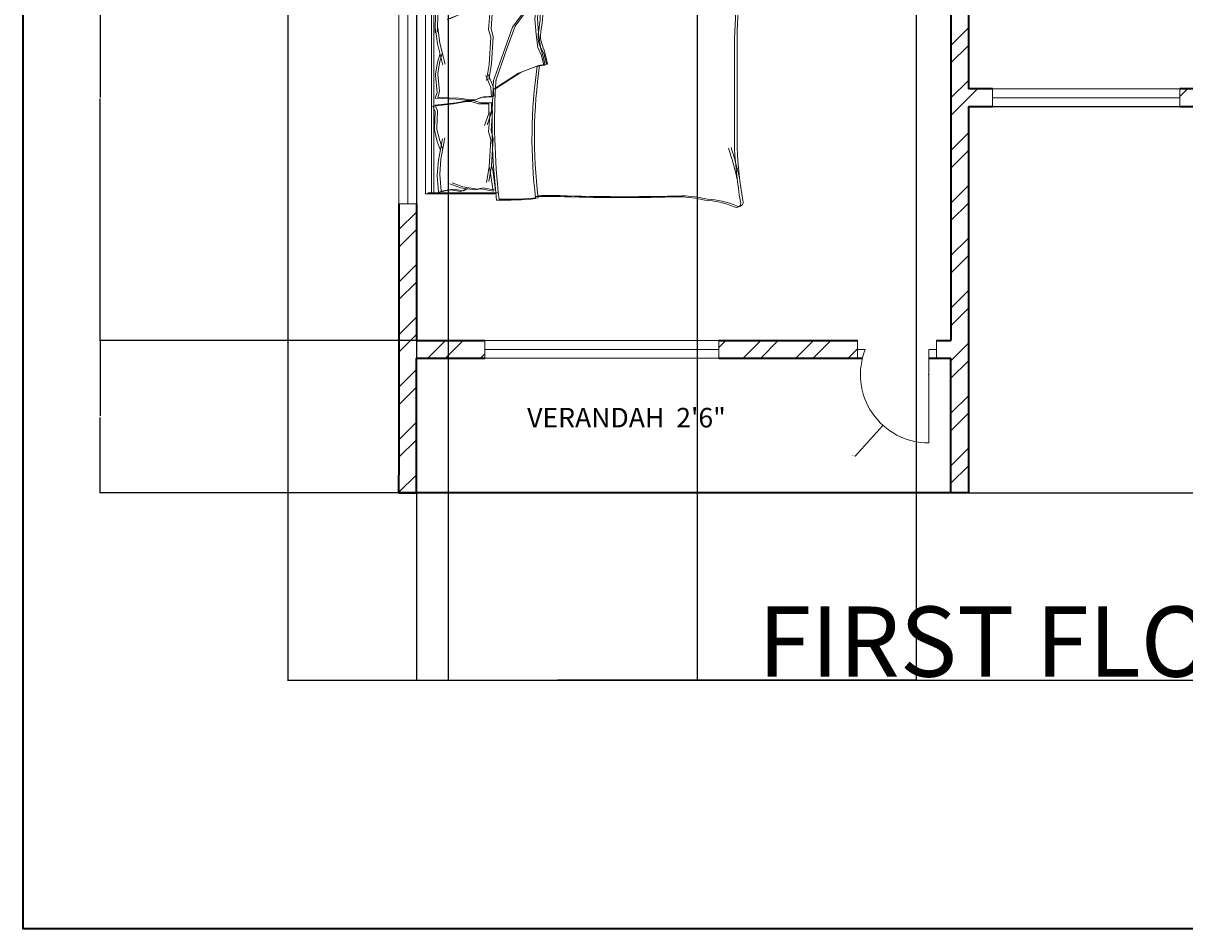
# Model space of a CAD drawing. Units: inches. Extents: x 2008 to 2657, y 1077 to 2165.
# Tile 1 of 16: x 2008 to 2306, y 1077 to 1309. Entities that reach past the tile are written whole.
import ezdxf

# ---------------------------------------------------------------- set-up
doc = ezdxf.new("R2010")
doc.units = ezdxf.units.IN
for name, color, linetype, lineweight in [('A-ANNO-DIMS', 2, 'Continuous', 18), ('A-ANNO-TITL', 7, 'Continuous', 35), ('A-ANNO-TTLB', 7, 'Continuous', 35), ('A-AREA-IDEN', 4, 'Continuous', 18), ('A-DOOR', 11, 'Continuous', 18), ('A-FURN', 8, 'Continuous', 13), ('A-GLAZ', 191, 'Continuous', 18), ('A-WALL', 7, 'Continuous', 35)]:
    doc.layers.add(name, color=color, linetype=linetype, lineweight=lineweight)
doc.layers.add('A-WALL-PATT', color=30, linetype='Continuous', lineweight=13, true_color=0xf8991e)
doc.styles.get("Standard").update_dxf_attribs({"font": 'arial.ttf'})
doc.dimstyles.get("Standard").update_dxf_attribs({"dimtxt": 0.18, "dimasz": 0.18, "dimexe": 0.18, "dimexo": 0.0625, "dimgap": 0.09, "dimtad": 0, "dimtih": 1, "dimtoh": 1, "dimdec": 4, "dimzin": 0, "dimdsep": 46, "dimtxsty": 'Standard', "dimcen": 0.09, "dimadec": 0, "dimazin": 0, "dimtfac": 1, "dimtdec": 4, "dimtofl": 0, "dimtmove": 0, "dimatfit": 3, "dimfxl": 1, "dimtolj": 1, "dimtzin": 0, "dimarcsym": 0})

# ---------------------------------------------------------------- blocks, each defined once
blk = doc.blocks.new('BED-DOUBLE')
for p, q in [((0, 51.49), (0.64, 51.49)), ((0, 3.48), (0, 51.49)), ((0, 51.27), (26.61, 51.27)), ((0, 51.27), (26.61, 51.27)), ((0.64, 51.49), (27.25, 51.49)), ((0.64, 51.49), (27.25, 51.49)), ((1.53, 3.48), (1.53, 51.27)), ((1.53, 3.48), (1.53, 51.27)), ((2.17, 3.7), (2.17, 51.49)), ((2.17, 3.7), (2.17, 51.49)), ((16.57, 50.7), (13.43, 49.92)), ((16.57, 50.7), (13.43, 49.92)), ((17.21, 50.93), (14.07, 50.15)), ((17.21, 50.93), (14.07, 50.15)), ((16.17, 45.57), (16.57, 50.7)), ((16.17, 45.57), (16.57, 50.7)), ((16.81, 45.8), (17.21, 50.93)), ((16.81, 45.8), (17.21, 50.93)), ((27.75, 52.87), (24.5, 49.16)), ((27.75, 52.87), (24.5, 49.16)), ((28.39, 53.1), (25.14, 49.39)), ((28.39, 53.1), (25.14, 49.39)), ((29.49, 52.95), (27.75, 52.87, 3.87)), ((29.49, 52.95), (27.75, 52.87, 3.87)), ((28.37, 51.33), (27.75, 52.87)), ((28.37, 51.33), (27.75, 52.87)), ((28.06, 48.23), (28.37, 51.33)), ((28.06, 48.23), (28.37, 51.33)), ((30.13, 53.18), (28.39, 53.1, 3.87)), ((30.13, 53.18), (28.39, 53.1, 3.87)), ((29, 51.56), (28.39, 53.1)), ((29, 51.56), (28.39, 53.1)), ((28.7, 48.46), (29, 51.56)), ((28.7, 48.46), (29, 51.56)), ((2.56, 50.11), (2.46, 44.71)), ((2.56, 50.11), (2.46, 44.71)), ((2.56, 50.11), (5.77, 49.73)), ((2.56, 50.11), (5.77, 49.73)), ((3.2, 50.34), (3.1, 44.94)), ((3.2, 50.34), (3.1, 44.94)), ((3.2, 50.34), (6.41, 49.96)), ((3.2, 50.34), (6.41, 49.96)), ((8.26, 49.31), (5.58, 48.13)), ((8.26, 49.31), (5.58, 48.13)), ((5.77, 49.73), (8.34, 50.33)), ((5.77, 49.73), (8.34, 50.33)), ((8.9, 49.54), (6.22, 48.36)), ((8.9, 49.54), (6.22, 48.36)), ((6.41, 49.96), (8.98, 50.56)), ((6.41, 49.96), (8.98, 50.56)), ((11.83, 50.11), (8.26, 49.31)), ((11.83, 50.11), (8.26, 49.31)), ((8.34, 50.33), (9.38, 49.82)), ((8.34, 50.33), (9.38, 49.81)), ((12.47, 50.34), (8.9, 49.54)), ((12.47, 50.34), (8.9, 49.54)), ((8.98, 50.56), (10.02, 50.04)), ((8.98, 50.56), (10.02, 50.04)), ((13.43, 49.92), (11.83, 50.11)), ((13.43, 49.92), (11.83, 50.11)), ((14.07, 50.15), (12.47, 50.34)), ((14.07, 50.15), (12.47, 50.34)), ((24.5, 49.16), (22.33, 46.22)), ((24.5, 49.16), (22.33, 46.22)), ((25.14, 49.39), (22.97, 46.45)), ((25.14, 49.39), (22.97, 46.45)), ((28.37, 44.36), (28.06, 48.23)), ((28.37, 44.36), (28.06, 48.23)), ((29, 44.59), (28.7, 48.46)), ((29, 44.59), (28.7, 48.46)), ((2.46, 44.71), (2.54, 45.71)), ((2.46, 44.71), (2.54, 45.71)), ((2.54, 45.71), (3.07, 41.91)), ((2.54, 45.71), (3.07, 41.91)), ((3.1, 44.94), (3.18, 45.94)), ((3.1, 44.94), (3.18, 45.94)), ((3.18, 45.94), (3.71, 42.14)), ((3.18, 45.94), (3.71, 42.14)), ((16.73, 43.61), (16.17, 45.57)), ((16.73, 43.61), (16.17, 45.57)), ((17.37, 43.84), (16.81, 45.8)), ((17.37, 43.83), (16.81, 45.8)), ((22.33, 46.22), (20.32, 40.64)), ((22.33, 46.22), (20.32, 40.64)), ((22.97, 46.45), (20.96, 40.87)), ((22.97, 46.45), (20.96, 40.87)), ((3.07, 41.91), (4.42, 36.5)), ((3.07, 41.91), (4.42, 36.5)), ((3.71, 42.14), (5.06, 36.72)), ((3.71, 42.14), (5.06, 36.72)), ((16.3, 36.6), (16.73, 43.61)), ((16.3, 36.6), (16.73, 43.61)), ((16.93, 36.83), (17.37, 43.84)), ((16.93, 36.82), (17.37, 43.83)), ((28.83, 40.95), (28.37, 44.36)), ((28.83, 40.95), (28.37, 44.36)), ((29.47, 41.18), (29, 44.59)), ((29.47, 41.18), (29, 44.59)), ((3.67, 39.2), (3.08, 37.14)), ((3.67, 39.2), (3.08, 37.14)), ((4.31, 39.43), (3.72, 37.36)), ((4.31, 39.43), (3.72, 37.36)), ((20.32, 40.64), (17.38, 32.31)), ((20.32, 40.64), (17.38, 32.31)), ((20.96, 40.87), (18.02, 32.54)), ((20.96, 40.87), (18.02, 32.53)), ((29.76, 38.94), (28.83, 40.95)), ((29.76, 38.94), (28.83, 40.95)), ((30.4, 39.17), (29.47, 41.18)), ((30.4, 39.17), (29.47, 41.18)), ((30.38, 36.46), (29.76, 38.94)), ((30.38, 36.46), (29.76, 38.94)), ((31.02, 36.69), (30.4, 39.17)), ((31.02, 36.69), (30.4, 39.17)), ((79.25, 15.06), (79.25, 39.68)), ((79.25, 15.06), (79.25, 39.68)), ((79.88, 15.29), (79.88, 39.91)), ((79.88, 15.29), (79.88, 39.91)), ((3.08, 37.14), (2.54, 34.21)), ((3.08, 37.14), (2.54, 34.2)), ((3.72, 37.36), (3.18, 34.43)), ((3.72, 37.36), (3.18, 34.43)), ((15.63, 32.56), (16.3, 36.6)), ((15.63, 32.56), (16.3, 36.6)), ((16.27, 32.79), (16.93, 36.83)), ((16.27, 32.79), (16.93, 36.82)), ((23.88, 34.45), (28.37, 36.15)), ((23.88, 34.45), (28.37, 36.15)), ((24.52, 34.68), (29, 36.38)), ((24.52, 34.68), (29, 36.38)), ((28.37, 36.15), (30.38, 36.46)), ((28.37, 36.15), (30.38, 36.46)), ((29, 36.38), (31.02, 36.69)), ((29, 36.38), (31.02, 36.69)), ((2.54, 34.21), (2.56, 33.88)), ((2.54, 34.2), (2.56, 33.88)), ((2.56, 33.88), (2.98, 29.46)), ((2.56, 33.88), (2.98, 29.46)), ((3.18, 34.43), (3.2, 34.11)), ((3.18, 34.43), (3.2, 34.11)), ((3.2, 34.11), (3.62, 29.68)), ((3.2, 34.11), (3.62, 29.68)), ((16.74, 30.75), (15.45, 33.82)), ((16.74, 30.75), (15.45, 33.82)), ((17.38, 30.98), (16.09, 34.05)), ((17.38, 30.98), (16.09, 34.05)), ((17.38, 30.26), (23.88, 34.45)), ((17.38, 30.26), (23.88, 34.45)), ((18.02, 30.49), (24.52, 34.68)), ((18.02, 30.49), (24.52, 34.68)), ((16.89, 28.3), (16.74, 30.75)), ((16.89, 28.3), (16.74, 30.75)), ((17.53, 28.53), (17.38, 30.98)), ((17.53, 28.53), (17.38, 30.98)), ((2.98, 29.46), (2.49, 27.98)), ((2.98, 29.46), (2.49, 27.98)), ((2.49, 27.98), (7.87, 27.73)), ((2.49, 27.98), (7.87, 27.73)), ((3.62, 29.68), (3.13, 28.21)), ((3.62, 29.68), (3.13, 28.21)), ((3.13, 28.21), (8.51, 27.96)), ((3.13, 28.21), (8.51, 27.96)), ((7.22, 26.56), (10.4, 27.14)), ((7.22, 26.56), (10.4, 27.14)), ((7.86, 26.79), (11.04, 27.37)), ((7.86, 26.79), (11.04, 27.37)), ((7.87, 27.73), (11.08, 27.36)), ((7.87, 27.73), (11.08, 27.36)), ((8.51, 27.96), (11.72, 27.58)), ((8.51, 27.96), (11.72, 27.58)), ((10.4, 27.14), (11.7, 27.14)), ((10.4, 27.14), (11.7, 27.14)), ((11.04, 27.37), (12.34, 27.37)), ((11.04, 27.37), (12.34, 27.37)), ((11.08, 27.36), (12.38, 27.44)), ((11.08, 27.36), (12.38, 27.44)), ((11.7, 27.14), (13.58, 26.56)), ((11.7, 27.14), (13.58, 26.56)), ((11.72, 27.58), (13.02, 27.66)), ((11.72, 27.58), (13.02, 27.66)), ((12.34, 27.37), (14.22, 26.79)), ((12.34, 27.37), (14.22, 26.79)), ((12.38, 27.44), (14.22, 28.13)), ((12.38, 27.44), (14.22, 28.13)), ((13.02, 27.66), (14.86, 28.36)), ((13.02, 27.66), (14.86, 28.36)), ((14.22, 28.13), (16.89, 28.3)), ((14.22, 28.13), (16.89, 28.3)), ((14.86, 28.36), (17.53, 28.53)), ((14.86, 28.36), (17.53, 28.53)), ((1.87, 25.98), (7.22, 26.56)), ((1.87, 25.98), (7.22, 26.56)), ((2.45, 24.54), (1.87, 25.98)), ((2.45, 24.54), (1.87, 25.98)), ((2.3, 20.09), (2.45, 24.54)), ((2.3, 20.09), (2.45, 24.54)), ((2.51, 26.21), (7.86, 26.79)), ((2.51, 26.21), (7.86, 26.79)), ((3.09, 24.77), (2.51, 26.21)), ((3.09, 24.77), (2.51, 26.21)), ((2.94, 20.32), (3.09, 24.77)), ((2.94, 20.32), (3.09, 24.77)), ((13.58, 26.56), (16.26, 26.56)), ((13.58, 26.56), (16.26, 26.56)), ((14.22, 26.79), (16.9, 26.79)), ((14.22, 26.79), (16.9, 26.79)), ((16.26, 24.1), (15.17, 20.96)), ((16.26, 24.1), (15.17, 20.96)), ((16.9, 24.33), (15.81, 21.19)), ((16.9, 24.33), (15.81, 21.19)), ((16.17, 19.38), (16.57, 24.52)), ((16.17, 19.38), (16.57, 24.52)), ((16.26, 26.56), (16.26, 24.1)), ((16.26, 26.56), (16.26, 24.1)), ((16.81, 19.61), (17.21, 24.74)), ((16.81, 19.61), (17.21, 24.74)), ((16.9, 26.79), (16.9, 24.33)), ((16.9, 26.79), (16.9, 24.33)), ((2.3, 19.77), (2.3, 20.09)), ((2.3, 19.77), (2.3, 20.09)), ((3.03, 16.88), (2.3, 19.77)), ((3.03, 16.88), (2.3, 19.77)), ((2.94, 20), (2.94, 20.32)), ((2.94, 20), (2.94, 20.32)), ((3.67, 17.11), (2.94, 20)), ((3.67, 17.11), (2.94, 20)), ((16.73, 17.42), (16.17, 19.38)), ((16.73, 17.42), (16.17, 19.38)), ((17.37, 17.65), (16.81, 19.61)), ((17.37, 17.65), (16.81, 19.61)), ((3.75, 14.86), (3.03, 16.88)), ((3.75, 14.86), (3.03, 16.88)), ((3.32, 12.11), (4.33, 17.6)), ((3.32, 12.11), (4.33, 17.6)), ((4.39, 15.08), (3.67, 17.11)), ((4.39, 15.08), (3.67, 17.11)), ((3.96, 12.34), (4.97, 17.83)), ((3.96, 12.34), (4.97, 17.83)), ((16.3, 10.41), (16.73, 17.42)), ((16.3, 10.41), (16.73, 17.42)), ((16.93, 10.64), (17.37, 17.65)), ((16.93, 10.64), (17.37, 17.65)), ((3.03, 8.29), (3.32, 12.11)), ((3.03, 8.29), (3.32, 12.11)), ((3.67, 8.51), (3.96, 12.34)), ((3.67, 8.51), (3.96, 12.34)), ((15.63, 6.38), (16.3, 10.41)), ((15.63, 6.38), (16.3, 10.41)), ((16.27, 6.61), (16.93, 10.64)), ((16.27, 6.61), (16.93, 10.64)), ((16.3, 10.41), (16.62, 9.28)), ((16.3, 10.41), (16.62, 9.28)), ((16.62, 9.28), (17.34, 4.18)), ((16.62, 9.28), (17.34, 4.18)), ((16.93, 10.64), (17.26, 9.51)), ((16.93, 10.64), (17.26, 9.51)), ((17.26, 9.51), (17.98, 4.41)), ((17.26, 9.51), (17.98, 4.41)), ((3.01, 8.18), (3.03, 8.29)), ((3.01, 8.18), (3.03, 8.29)), ((3.34, 3.9), (3.01, 8.18)), ((3.34, 3.9), (3.01, 8.18)), ((3.65, 8.41), (3.67, 8.51)), ((3.65, 8.41), (3.67, 8.51)), ((3.98, 4.13), (3.65, 8.41)), ((3.98, 4.13), (3.65, 8.41)), ((8.96, 5.05), (6.21, 6.06)), ((8.96, 5.05), (6.21, 6.06)), ((9.59, 5.28), (6.85, 6.29)), ((9.59, 5.28), (6.85, 6.29)), ((18.11, 3.48), (0, 3.48)), ((18.11, 3.48), (0, 3.48)), ((18.75, 3.7), (0.64, 3.7)), ((18.75, 3.7), (0.64, 3.7)), ((3.32, 3.9), (6.5, 4.47)), ((3.32, 3.89), (6.5, 4.47)), ((3.96, 4.12), (7.14, 4.7)), ((3.96, 4.12), (7.14, 4.7)), ((6.5, 4.47), (9.1, 4.04)), ((6.5, 4.47), (9.1, 4.04)), ((7.14, 4.7), (9.74, 4.27)), ((7.14, 4.7), (9.74, 4.27)), ((12.57, 4.47), (8.96, 5.05)), ((12.57, 4.47), (8.96, 5.05)), ((9.1, 4.04), (10.11, 4.62)), ((9.1, 4.04), (10.11, 4.62)), ((13.21, 4.7), (9.59, 5.28)), ((13.21, 4.7), (9.59, 5.28)), ((9.74, 4.27), (10.75, 4.85)), ((9.74, 4.27), (10.75, 4.85)), ((14.16, 4.76), (12.57, 4.47)), ((14.16, 4.76), (12.57, 4.47)), ((14.8, 4.99), (13.21, 4.7)), ((14.8, 4.99), (13.21, 4.7)), ((17.34, 4.18), (14.16, 4.76)), ((17.34, 4.18), (14.16, 4.76)), ((17.98, 4.41), (14.8, 4.99)), ((17.98, 4.41), (14.8, 4.99))]:
    blk.add_line(p, q)
for centre, radius, start, end in [((68.67, 76.16), 23.07, 267.4714, 296.4681), ((68.67, 76.16), 23.07, 267.4714, 296.4681), ((69.31, 76.39), 23.07, 267.4714, 296.4681), ((69.31, 76.39), 23.07, 267.4714, 296.4681), ((78.87, 54.41), 1.1, 332.6588, 86.02), ((78.87, 54.41), 1.1, 332.6588, 86.02), ((212.28, 41.15), 133.04, 174.4998, 180.6351), ((212.28, 41.15), 133.04, 174.4998, 180.6351), ((79.51, 54.64), 1.1, 332.6588, 86.02), ((79.51, 54.64), 1.1, 332.6588, 86.02), ((212.92, 41.38), 133.04, 174.4998, 180.6351), ((212.92, 41.38), 133.04, 174.4998, 180.6351), ((-6.66, 51.33), 36.18, 349.8763, 2.5657), ((-6.66, 51.33), 36.18, 349.8763, 2.5657), ((36.32, 182.27), 129.5, 266.9791, 273.8365), ((36.32, 182.27), 129.5, 266.9791, 273.8365), ((-6.02, 51.56), 36.18, 349.8763, 2.5657), ((-6.02, 51.56), 36.18, 349.8763, 2.5657), ((36.95, 182.49), 129.5, 266.9791, 273.8365), ((36.95, 182.49), 129.5, 266.9791, 273.8365), ((67.82, -4508.74), 4561.86, 90.00217, 90.28689), ((67.82, -4508.74), 4561.86, 90.00217, 90.28689), ((68.46, -4508.51), 4561.86, 90.00217, 90.28689), ((68.46, -4508.51), 4561.86, 90.00217, 90.28689), ((35.07, 43.74), 6.22, 168.6608, 203.7384), ((35.07, 43.74), 6.22, 168.6608, 203.7384), ((35.71, 43.97), 6.22, 168.6608, 203.7384), ((35.71, 43.97), 6.22, 168.6608, 203.7384), ((1.48, 31.15), 29.65, 10.6617, 19.8806), ((1.48, 31.15), 29.65, 10.6617, 19.8806), ((2.12, 31.38), 29.65, 10.6617, 19.8806), ((2.12, 31.38), 29.65, 10.6617, 19.8806), ((156.32, 17.76), 129.02, 171.7845, 186.9006), ((156.32, 17.76), 129.02, 171.7845, 186.9006), ((156.96, 17.98), 129.02, 171.7845, 186.9006), ((156.96, 17.98), 129.02, 171.7845, 186.9006), ((30.44, 36.64), 0.185, 250.2464, 1.1377), ((30.44, 36.64), 0.185, 250.2464, 1.1377), ((31.08, 36.87), 0.185, 250.2464, 1.1377), ((31.08, 36.86), 0.185, 250.2464, 1.1377), ((182.69, 21.59), 164.97, 176.0865, 186.7821), ((182.69, 21.59), 164.97, 176.0865, 186.7821), ((182.05, 21.36), 164.97, 176.0865, 186.7821), ((182.05, 21.36), 164.97, 176.0865, 186.7821), ((-23.71, -17.22), 106.46, 13.3832, 17.7053), ((-23.71, -17.22), 106.46, 13.3832, 17.7053), ((-23.07, -16.99), 106.46, 13.3832, 17.7053), ((-23.07, -16.99), 106.46, 13.3832, 17.7053), ((200.84, 21.43), 121.76, 182.9958, 189.4091), ((200.84, 21.43), 121.76, 182.9958, 189.4091), ((201.48, 21.66), 121.76, 182.9958, 189.4091), ((201.48, 21.66), 121.76, 182.9958, 189.4091), ((31.81, -167.08), 170.11, 88.4762, 91.0082), ((31.81, -167.08), 170.11, 88.4762, 91.0082), ((20.1, 85.16), 83.31, 268.7218, 275.604), ((20.1, 85.16), 83.31, 268.7218, 275.604), ((20.74, 85.39), 83.31, 268.7218, 275.604), ((20.74, 85.39), 83.31, 268.7218, 275.604), ((31.17, -167.31), 170.11, 88.4762, 91.0082), ((31.17, -167.31), 170.11, 88.4762, 91.0082), ((50.61, 484.82), 482.31, 268.2277, 271.7185), ((50.61, 484.82), 482.31, 268.2277, 271.7185), ((51.25, 485.05), 482.31, 268.2277, 271.7185), ((51.25, 485.05), 482.31, 268.2277, 271.7185), ((64.52, -26.9), 29.63, 76.0648, 88.9113), ((64.52, -26.9), 29.63, 76.0648, 88.9113), ((65.15, -26.67), 29.63, 76.0648, 88.9113), ((65.15, -26.67), 29.63, 76.0648, 88.9113), ((70.28, -21.66), 23.56, 67.9751, 86.652), ((70.28, -21.66), 23.56, 67.9751, 86.652), ((70.92, -21.43), 23.56, 67.9751, 86.652), ((70.92, -21.43), 23.56, 67.9751, 86.652), ((79.72, 1.09), 1.09, 236.1736, 23.4781), ((79.72, 1.09), 1.09, 236.1736, 23.4781), ((80.36, 1.32), 1.09, 236.1736, 23.4781), ((80.36, 1.32), 1.09, 236.1736, 23.4781)]:
    blk.add_arc(centre, radius, start, end)
blk = doc.blocks.new('WIN-60IN-B')
for p, q in [((0, 4.5), (0, 0)), ((0, 4.5), (60, 4.5)), ((60, 2.25), (60, 4.5)), ((60, 4.5), (60, 0)), ((0, 0), (0, 2.25)), ((0, 2.25), (60, 2.25)), ((60, 0), (0, 0))]:
    blk.add_line(p, q)
blk = doc.blocks.new('WIN-60IN-A')
for p, q in [((0, 60), (4.5, 60)), ((0, 60), (0, 0)), ((4.5, 60), (2.25, 60)), ((2.25, 60), (2.25, 0)), ((4.5, 0), (4.5, 60)), ((4.5, 0), (0, 0)), ((2.25, 0), (4.5, 0))]:
    blk.add_line(p, q)
blk = doc.blocks.new('*D31')
at = {"layer": 'A-ANNO-DIMS', "color": 0, "lineweight": -2, "transparency": 16777216}
for p, q in [((2076.26, 1562.18), (2076.26, 1140.44)), ((2576.76, 1188.61), (2576.76, 1140.44)), ((2076.44, 1140.62), (2326.12, 1140.62)), ((2576.58, 1140.62), (2326.91, 1140.62))]:
    blk.add_line(p, q, dxfattribs=at)
at = {"layer": 'A-ANNO-DIMS', "color": 0, "transparency": 16777216}
for points in [[(2076.44, 1140.65), (2076.44, 1140.59), (2076.26, 1140.62)], [(2576.58, 1140.65), (2576.58, 1140.59), (2576.76, 1140.62)]]:
    blk.add_solid(points, dxfattribs=at)
at = {"layer": 'Defpoints', "color": 0, "transparency": 16777216}
for p in [(2076.26, 1562.24), (2576.76, 1188.67), (2576.76, 1140.62)]:
    blk.add_point(p, dxfattribs=at)
at = {"layer": 'A-ANNO-DIMS', "color": 0, "transparency": 16777216, "insert": (2326.51, 1140.62), "char_height": 0.18, "attachment_point": 5}
blk.add_mtext('\\A1;500.5', dxfattribs=at)
blk = doc.blocks.new('*D38')
at = {"layer": 'A-ANNO-DIMS', "color": 0, "lineweight": -2, "transparency": 16777216}
for p, q in [((2109.2, 1227.67), (2028.03, 1227.67)), ((2028.21, 1227.49), (2028.21, 1208.36)), ((2028.21, 1188.85), (2028.21, 1207.99)), ((2104.7, 1188.67), (2028.03, 1188.67))]:
    blk.add_line(p, q, dxfattribs=at)
at = {"layer": 'A-ANNO-DIMS', "color": 0, "transparency": 16777216}
for points in [[(2028.18, 1227.49), (2028.24, 1227.49), (2028.21, 1227.67)], [(2028.18, 1188.85), (2028.24, 1188.85), (2028.21, 1188.67)]]:
    blk.add_solid(points, dxfattribs=at)
at = {"layer": 'Defpoints', "color": 0, "transparency": 16777216}
for p in [(2028.21, 1227.67), (2109.26, 1227.67), (2104.76, 1188.67)]:
    blk.add_point(p, dxfattribs=at)
at = {"layer": 'A-ANNO-DIMS', "color": 0, "transparency": 16777216, "insert": (2028.21, 1208.17), "char_height": 0.18, "attachment_point": 5}
blk.add_mtext('\\A1;39', dxfattribs=at)
blk = doc.blocks.new('*D39')
at = {"layer": 'A-ANNO-DIMS', "color": 0, "lineweight": -2, "transparency": 16777216}
for p, q in [((2109.2, 1352.17), (2028.03, 1352.17)), ((2028.21, 1351.99), (2028.21, 1290.11)), ((2028.21, 1227.85), (2028.21, 1289.74)), ((2109.2, 1227.67), (2028.03, 1227.67))]:
    blk.add_line(p, q, dxfattribs=at)
at = {"layer": 'A-ANNO-DIMS', "color": 0, "transparency": 16777216}
for points in [[(2028.18, 1351.99), (2028.24, 1351.99), (2028.21, 1352.17)], [(2028.18, 1227.85), (2028.24, 1227.85), (2028.21, 1227.67)]]:
    blk.add_solid(points, dxfattribs=at)
at = {"layer": 'Defpoints', "color": 0, "transparency": 16777216}
for p in [(2028.21, 1352.17), (2109.26, 1352.17), (2109.26, 1227.67)]:
    blk.add_point(p, dxfattribs=at)
at = {"layer": 'A-ANNO-DIMS', "color": 0, "transparency": 16777216, "insert": (2028.21, 1289.92), "char_height": 0.18, "attachment_point": 5}
blk.add_mtext('\\A1;124.5', dxfattribs=at)
blk = doc.blocks.new('*D50')
at = {"layer": 'A-ANNO-DIMS', "color": 0, "lineweight": -2, "transparency": 16777216}
for p, q in [((2250.82, 1287.67), (2624.99, 1287.67)), ((2624.81, 1287.49), (2624.81, 1238.36)), ((2624.81, 1188.85), (2624.81, 1237.99)), ((2250.82, 1188.67), (2624.99, 1188.67))]:
    blk.add_line(p, q, dxfattribs=at)
at = {"layer": 'A-ANNO-DIMS', "color": 0, "transparency": 16777216}
for points in [[(2624.78, 1287.49), (2624.84, 1287.49), (2624.81, 1287.67)], [(2624.78, 1188.85), (2624.84, 1188.85), (2624.81, 1188.67)]]:
    blk.add_solid(points, dxfattribs=at)
at = {"layer": 'Defpoints', "color": 0, "transparency": 16777216}
for p in [(2250.76, 1287.67), (2624.81, 1287.67), (2250.76, 1188.67)]:
    blk.add_point(p, dxfattribs=at)
at = {"layer": 'A-ANNO-DIMS', "color": 0, "transparency": 16777216, "insert": (2624.81, 1238.17), "char_height": 0.18, "attachment_point": 5}
blk.add_mtext('\\A1;99', dxfattribs=at)
blk = doc.blocks.new('*D55')
at = {"layer": 'A-ANNO-DIMS', "color": 0, "lineweight": -2, "transparency": 16777216}
for p, q in [((2109.26, 1509.68), (2109.26, 1140.44)), ((2181.26, 1509.68), (2181.26, 1140.44)), ((2109.44, 1140.62), (2145.04, 1140.62)), ((2181.08, 1140.62), (2145.48, 1140.62))]:
    blk.add_line(p, q, dxfattribs=at)
at = {"layer": 'A-ANNO-DIMS', "color": 0, "transparency": 16777216}
for points in [[(2109.44, 1140.65), (2109.44, 1140.59), (2109.26, 1140.62)], [(2181.08, 1140.65), (2181.08, 1140.59), (2181.26, 1140.62)]]:
    blk.add_solid(points, dxfattribs=at)
at = {"layer": 'Defpoints', "color": 0, "transparency": 16777216}
for p in [(2109.26, 1509.74), (2181.26, 1509.74), (2109.26, 1140.62)]:
    blk.add_point(p, dxfattribs=at)
at = {"layer": 'A-ANNO-DIMS', "color": 0, "transparency": 16777216, "insert": (2145.26, 1140.62), "char_height": 0.18, "attachment_point": 5}
blk.add_mtext('\\A1;72', dxfattribs=at)
blk = doc.blocks.new('*D62')
at = {"layer": 'A-ANNO-DIMS', "color": 0, "lineweight": -2, "transparency": 16777216}
for p, q in [((2117.38, 1566.68), (2117.38, 1140.44)), ((2237.38, 1566.68), (2237.38, 1140.44)), ((2117.56, 1140.62), (2177.1, 1140.62)), ((2237.2, 1140.62), (2177.66, 1140.62))]:
    blk.add_line(p, q, dxfattribs=at)
at = {"layer": 'A-ANNO-DIMS', "color": 0, "transparency": 16777216}
for points in [[(2117.56, 1140.65), (2117.56, 1140.59), (2117.38, 1140.62)], [(2237.2, 1140.65), (2237.2, 1140.59), (2237.38, 1140.62)]]:
    blk.add_solid(points, dxfattribs=at)
at = {"layer": 'Defpoints', "color": 0, "transparency": 16777216}
for p in [(2117.38, 1566.74), (2237.38, 1566.74), (2237.38, 1140.62)]:
    blk.add_point(p, dxfattribs=at)
at = {"layer": 'A-ANNO-DIMS', "color": 0, "transparency": 16777216, "insert": (2177.38, 1140.62), "char_height": 0.18, "attachment_point": 5}
blk.add_mtext('\\A1;120', dxfattribs=at)
blk = doc.blocks.new('*D97')
at = {"layer": 'A-ANNO-DIMS', "color": 0, "lineweight": -2, "transparency": 16777216}
for p, q in [((2240.52, 1218.95), (2240.7, 1218.95)), ((2240.61, 1218.86), (2240.61, 1219.04)), ((2221.82, 1198.14), (2228.74, 1205.81)), ((2221.64, 1198.14), (2221.82, 1198.14))]:
    blk.add_line(p, q, dxfattribs=at)
at = {"layer": 'A-ANNO-DIMS', "color": 0, "transparency": 16777216}
blk.add_solid([(2228.72, 1205.83), (2228.76, 1205.79), (2228.86, 1205.94)], dxfattribs=at)
at = {"layer": 'Defpoints', "color": 0, "transparency": 16777216}
for p in [(2240.61, 1218.95), (2228.86, 1205.94)]:
    blk.add_point(p, dxfattribs=at)
at = {"layer": 'A-ANNO-DIMS', "color": 0, "transparency": 16777216, "insert": (2221.16, 1198.14), "char_height": 0.18, "attachment_point": 5}
blk.add_mtext('\\A1;R17.52', dxfattribs=at)

msp = doc.modelspace()

# ---------------------------------------------------------------- hatches: boundary and pattern name
at = {"layer": 'A-WALL-PATT'}
h = msp.add_hatch(dxfattribs=at)
h.set_pattern_fill('ANSI32', color=256)
h.paths.add_polyline_path([(2109.2619, 2094.6743), (2104.7619, 2094.6743), (2104.7619, 2072.1743), (2104.7619, 2021.6151), (2109.2619, 2021.6151), (2109.2619, 2055.6743), (2126.1387, 2055.6743), (2126.1387, 2057.9243), (2126.1387, 2060.1743), (2109.2619, 2060.1743)])
h.paths.add_polyline_path([(2223.2494, 2057.9243), (2223.2494, 2060.1743), (2186.1387, 2060.1743), (2186.1387, 2055.6743), (2223.2494, 2055.6743)])
h.paths.add_polyline_path([(2250.7619, 2072.1743), (2250.7619, 2090.1743), (2250.7619, 2094.6743), (2246.2619, 2094.6743), (2246.2619, 2060.1743), (2242.7242, 2060.1743), (2242.7242, 2055.6743), (2246.2619, 2055.6743), (2246.2619, 1899.6743), (2242.7458, 1899.6743), (2242.7458, 1897.4243), (2242.7458, 1895.1743), (2246.2619, 1895.1743), (2246.2619, 1878.8745), (2248.5119, 1878.8745), (2250.7619, 1878.8745), (2250.7619, 1991.1743), (2250.7619, 2025.6743), (2257.6798, 2025.6743), (2257.6798, 2027.9243), (2257.6798, 2030.1743), (2250.7619, 2030.1743)])
h.paths.add_polyline_path([(2411.2619, 2031.6743), (2409.0119, 2031.6743), (2406.7619, 2031.6743), (2406.7619, 2030.1743), (2322.7619, 2030.1743), (2322.7619, 2053.3443), (2318.2619, 2053.3443), (2318.2619, 2030.1743), (2305.6798, 2030.1743), (2305.6798, 2025.6743), (2318.2619, 2025.6743), (2322.7619, 2025.6743), (2406.7619, 2025.6743), (2406.7619, 1995.6743), (2406.7619, 1847.2677), (2250.7619, 1847.2677), (2250.7619, 1850.9902), (2248.5119, 1850.9902), (2246.2619, 1850.9902), (2246.2619, 1847.1743), (2246.2619, 1842.7677), (2303.0015, 1842.7677), (2303.0015, 1667.2413), (2298.4208, 1667.2413), (2298.4208, 1662.7413), (2303.0015, 1662.7413), (2303.0015, 1649.8758), (2307.5015, 1649.8758), (2307.5015, 1842.7677), (2406.7619, 1842.7677), (2411.2619, 1842.7677), (2411.2619, 1878.6743), (2415.8196, 1878.6743), (2415.8196, 1880.9243), (2415.8196, 1883.1743), (2411.2619, 1883.1743)])
h.paths.add_polyline_path([(2411.2619, 2094.6743), (2406.7619, 2094.6743), (2318.2619, 2094.6743), (2318.2619, 2077.3443), (2322.7619, 2077.3443), (2322.7619, 2090.1743), (2406.7619, 2090.1743), (2406.7619, 2072.1743), (2406.7619, 2067.6743), (2406.7619, 2052.7524), (2411.2619, 2052.7524), (2411.2619, 2055.6743), (2414.9888, 2055.6743), (2414.9888, 2057.9243), (2414.9888, 2060.1743), (2411.2619, 2060.1743), (2411.2619, 2072.1743)])
h.paths.add_polyline_path([(2576.7619, 2072.1743), (2576.7619, 2094.6743), (2572.2619, 2094.6743), (2572.2619, 2060.1743), (2525.8113, 2060.1743), (2525.8113, 2055.6743), (2572.2619, 2055.6743), (2572.2619, 1994.289), (2576.7619, 1994.289)])
h.paths.add_polyline_path([(2465.8113, 2060.1743), (2436.2802, 2060.1743), (2436.2802, 2055.6743), (2465.8113, 2055.6743), (2465.8113, 2057.9243)])
h.paths.add_polyline_path([(2576.7619, 1934.289), (2574.5119, 1934.289), (2572.2619, 1934.289), (2572.2619, 1883.1743), (2447.7027, 1883.1743), (2447.7027, 1878.6743), (2459.7619, 1878.6743), (2459.7619, 1830.4982), (2464.2619, 1830.4982), (2464.2619, 1878.6743), (2572.2619, 1878.6743), (2572.2619, 1868.4883), (2576.7619, 1868.4883)])
h.paths.add_polyline_path([(2576.7619, 1832.4883), (2572.2619, 1832.4883), (2572.2619, 1806.6743), (2464.2619, 1806.6743), (2464.2619, 1809.6629), (2459.7619, 1809.6629), (2459.7619, 1802.1743), (2483.7619, 1802.1743), (2483.7619, 1778.1743), (2488.2619, 1778.1743), (2488.2619, 1802.1743), (2572.2619, 1802.1743), (2572.2619, 1793.6101), (2576.7619, 1793.6101)])
h.paths.add_polyline_path([(2576.7619, 1769.6101), (2572.2619, 1769.6101), (2572.2619, 1754.1743), (2488.2619, 1754.1743), (2488.2619, 1757.2675), (2486.0119, 1757.2675), (2483.7619, 1757.2675), (2483.7619, 1754.1743), (2447.4528, 1754.1743), (2447.4528, 1749.6743), (2483.7619, 1749.6743), (2572.2619, 1749.6743), (2572.2619, 1715.1837), (2576.7619, 1715.1837)])
h.paths.add_polyline_path([(2576.7619, 1655.1837), (2572.2619, 1655.1837), (2572.2619, 1617.6743), (2411.2619, 1617.6743), (2411.2619, 1749.6743), (2414.2827, 1749.6743), (2414.2827, 1754.1743), (2406.7619, 1754.1743), (2406.7619, 1749.6743), (2406.7619, 1617.6743), (2307.5015, 1617.6743), (2307.5015, 1621.0007), (2305.2515, 1621.0007), (2303.0015, 1621.0007), (2303.0015, 1609.6944), (2307.5015, 1609.6944), (2307.5015, 1613.1743), (2406.7619, 1613.1743), (2406.7619, 1476.6743), (2415.532, 1476.6743), (2415.532, 1478.9243), (2415.532, 1481.1743), (2411.2619, 1481.1743), (2411.2619, 1613.1743), (2572.2619, 1613.1743), (2572.2619, 1584.6086), (2576.7619, 1584.6086)])
h.paths.add_polyline_path([(2576.7619, 1524.6086), (2572.2619, 1524.6086), (2572.2619, 1481.1743), (2483.7619, 1481.1743), (2447.5119, 1481.1743), (2447.5119, 1476.6743), (2483.7619, 1476.6743), (2483.7619, 1473.5051), (2488.2619, 1473.5051), (2488.2619, 1476.6743), (2572.2619, 1476.6743), (2572.2619, 1469.5488), (2576.7619, 1469.5488)])
h.paths.add_polyline_path([(2576.7619, 1445.5488), (2572.2619, 1445.5488), (2572.2619, 1428.6743), (2488.2619, 1428.6743), (2488.2619, 1455.6743), (2486.0119, 1455.6743), (2483.7619, 1455.6743), (2483.7619, 1428.6743), (2459.7619, 1428.6743), (2459.7619, 1422.1519), (2464.2619, 1422.1519), (2464.2619, 1424.1743), (2572.2619, 1424.1743), (2572.2619, 1407.5685), (2576.7619, 1407.5685)])
h.paths.add_polyline_path([(2576.7619, 1371.5685), (2572.2619, 1371.5685), (2572.2619, 1352.1743), (2464.2619, 1352.1743), (2464.2619, 1403.1384), (2462.0119, 1403.1384), (2459.7619, 1403.1384), (2459.7619, 1352.1743), (2446.3194, 1352.1743), (2446.3194, 1347.6743), (2572.2619, 1347.6743), (2572.2619, 1321.0291), (2576.7619, 1321.0291)])
h.paths.add_polyline_path([(2462.703, 1227.6743), (2436.0298, 1227.6743), (2436.0298, 1225.4243), (2436.0298, 1223.1743), (2462.703, 1223.1743), (2462.703, 1225.4243)])
h.paths.add_polyline_path([(2576.7619, 1261.0291), (2574.5119, 1261.0291), (2572.2619, 1261.0291), (2572.2619, 1227.6743), (2522.703, 1227.6743), (2522.703, 1223.1743), (2572.2619, 1223.1743), (2572.2619, 1188.6743), (2576.7619, 1188.6743), (2576.7619, 1193.1743), (2576.7619, 1223.1743)])
h.paths.add_polyline_path([(2414.2823, 1227.6743), (2411.2619, 1227.6743), (2411.2619, 1267.1779), (2409.0119, 1267.1779), (2406.7619, 1267.1779), (2406.7619, 1227.6743), (2322.7619, 1227.6743), (2322.7619, 1244.3623), (2318.2619, 1244.3623), (2318.2619, 1223.1743), (2406.7619, 1223.1743), (2406.7619, 1193.1743), (2406.7619, 1188.6743), (2411.2619, 1188.6743), (2411.2619, 1193.1743), (2411.2619, 1223.1743), (2414.2823, 1223.1743)])
h.paths.add_polyline_path([(2411.2619, 1347.6743), (2414.702, 1347.6743), (2414.702, 1349.9243), (2414.702, 1352.1743), (2411.2619, 1352.1743), (2411.2619, 1416.7413), (2307.5015, 1416.7413), (2307.5015, 1579.8489), (2305.2515, 1579.8489), (2303.0015, 1579.8489), (2303.0015, 1566.7413), (2299.2719, 1566.7413), (2299.2719, 1562.2413), (2303.0015, 1562.2413), (2303.0015, 1416.7413), (2246.2619, 1416.7413), (2246.2619, 1409.8616), (2250.7619, 1409.8616), (2250.7619, 1412.2413), (2406.7619, 1412.2413), (2406.7619, 1292.1743), (2304.9703, 1292.1743), (2304.9703, 1287.6743), (2318.2619, 1287.6743), (2318.2619, 1268.3623), (2322.7619, 1268.3623), (2322.7619, 1287.6743), (2406.7619, 1287.6743), (2406.7619, 1285.4748), (2411.2619, 1285.4748)])
h.paths.add_polyline_path([(2109.2619, 1262.7482), (2104.7619, 1262.7482), (2104.7619, 1223.1743), (2104.7619, 1193.1743), (2104.7619, 1188.6743), (2109.2619, 1188.6743), (2109.2619, 1223.1743), (2126.7928, 1223.1743), (2126.7928, 1225.4243), (2126.7928, 1227.6743), (2109.2619, 1227.6743)])
h.paths.add_polyline_path([(2222.3268, 1227.6743), (2186.7928, 1227.6743), (2186.7928, 1223.1743), (2222.3268, 1223.1743)])
h.paths.add_polyline_path([(2250.7619, 1287.6743), (2256.9703, 1287.6743), (2256.9703, 1289.9243), (2256.9703, 1292.1743), (2250.7619, 1292.1743), (2250.7619, 1382.2078), (2248.5119, 1382.2078), (2246.2619, 1382.2078), (2246.2619, 1347.6743), (2246.2619, 1227.6743), (2242.6068, 1227.6743), (2242.6068, 1223.1743), (2246.2619, 1223.1743), (2246.2619, 1188.6743), (2250.7619, 1188.6743), (2250.7619, 1193.1743), (2250.7619, 1227.6743)])
h.paths.add_polyline_path([(2133.2619, 1349.9243), (2133.2619, 1352.1743), (2109.2619, 1352.1743), (2109.2619, 1375.2826), (2104.7619, 1375.2826), (2104.7619, 1322.7482), (2109.2619, 1322.7482), (2109.2619, 1347.6743), (2133.2619, 1347.6743)])
h.paths.add_polyline_path([(2210.2105, 1352.1743), (2161.7619, 1352.1743), (2161.7619, 1412.2413), (2185.7619, 1412.2413), (2185.7619, 1420.1851), (2183.5119, 1420.1851), (2181.2619, 1420.1851), (2181.2619, 1416.7413), (2109.2619, 1416.7413), (2109.2619, 1452.4006), (2104.7619, 1452.4006), (2104.7619, 1399.2826), (2109.2619, 1399.2826), (2109.2619, 1412.2413), (2157.2619, 1412.2413), (2157.2619, 1352.1743), (2154.3383, 1352.1743), (2154.3383, 1347.6743), (2210.2105, 1347.6743)])
h.paths.add_polyline_path([(2185.7619, 1514.2413), (2161.7619, 1514.2413), (2161.7619, 1518.1307), (2159.5119, 1518.1307), (2157.2619, 1518.1307), (2157.2619, 1514.2413), (2109.2619, 1514.2413), (2109.2619, 1528.997), (2107.0119, 1528.997), (2104.7619, 1528.997), (2104.7619, 1488.4006), (2109.2619, 1488.4006), (2109.2619, 1509.7413), (2181.2619, 1509.7413), (2181.2619, 1441.2042), (2185.7619, 1441.2042)])
h.paths.add_polyline_path([(2270.4025, 1566.7413), (2109.2619, 1566.7413), (2080.7619, 1566.7413), (2080.7619, 1586.5643), (2076.2619, 1586.5643), (2076.2619, 1562.2413), (2080.7619, 1562.2413), (2104.7619, 1562.2413), (2104.7619, 1552.997), (2109.2619, 1552.997), (2109.2619, 1562.2413), (2157.2619, 1562.2413), (2157.2619, 1538.2413), (2161.7619, 1538.2413), (2161.7619, 1562.2413), (2205.2619, 1562.2413), (2270.4025, 1562.2413)])
h.paths.add_polyline_path([(2131.6813, 1897.4243), (2131.6813, 1899.6743), (2109.2619, 1899.6743), (2109.2619, 1961.6151), (2104.7619, 1961.6151), (2104.7619, 1886.8042), (2109.2619, 1886.8042), (2109.2619, 1895.1743), (2131.6813, 1895.1743)])
h.paths.add_polyline_path([(2185.7619, 1847.1743), (2161.7619, 1847.1743), (2161.7619, 1895.1743), (2185.7619, 1895.1743), (2211.543, 1895.1743), (2211.543, 1897.4243), (2211.543, 1899.6743), (2154.0916, 1899.6743), (2154.0916, 1897.4243), (2154.0916, 1895.1743), (2157.2619, 1895.1743), (2157.2619, 1847.1743), (2109.2619, 1847.1743), (2109.2619, 1862.8042), (2104.7619, 1862.8042), (2104.7619, 1821.243), (2109.2619, 1821.243), (2109.2619, 1842.6743), (2181.2619, 1842.6743), (2181.2619, 1840.6763), (2185.7619, 1840.6763)])
h.paths.add_polyline_path([(2109.2619, 1785.243), (2104.7619, 1785.243), (2104.7619, 1715.4691), (2109.2619, 1715.4691), (2109.2619, 1730.8423), (2157.2619, 1730.8423), (2157.2619, 1727.6404), (2161.7619, 1727.6404), (2161.7619, 1730.8423), (2185.7619, 1730.8423), (2185.7619, 1822.1438), (2183.5119, 1822.1438), (2181.2619, 1822.1438), (2181.2619, 1735.3423), (2109.2619, 1735.3423)])
h.paths.add_polyline_path([(2109.2619, 1691.4691), (2104.7619, 1691.4691), (2104.7619, 1667.2413), (2076.2619, 1667.2413), (2076.2619, 1646.5643), (2080.7619, 1646.5643), (2080.7619, 1662.7413), (2109.2619, 1662.7413), (2271.4941, 1662.7413), (2271.4941, 1664.9913), (2271.4941, 1667.2413), (2181.2619, 1667.2413), (2161.7619, 1667.2413), (2161.7619, 1708.3752), (2159.5119, 1708.3752), (2157.2619, 1708.3752), (2157.2619, 1667.2413), (2109.2619, 1667.2413)])
h.paths.add_polyline_path([(2233.1467, 1747.4973), (2270.0737, 1747.4973), (2270.0737, 1766.1547), (2233.1467, 1766.1547)], flags=9)

# ---------------------------------------------------------------- linework, layer by layer
at = {"layer": 'A-ANNO-TTLB'}
msp.add_lwpolyline([(2008.4537, 2164.5615), (2657.4477, 2164.5615), (2657.4477, 1076.8888), (2008.4537, 1076.8888)], close=True, dxfattribs=at)
at = {"layer": 'A-DOOR'}
for p, q in [((2222.3268, 1223.1743), (2222.3268, 1227.6743)), ((2222.3268, 1227.6743), (2222.3268, 1225.4243)), ((2242.6068, 1227.6743), (2242.6068, 1223.1743)), ((2222.3268, 1225.4243), (2224.3268, 1225.4243)), ((2242.6068, 1225.4243), (2240.6068, 1225.4243)), ((2240.6068, 1225.4243), (2240.6068, 1201.4243)), ((2242.6068, 1223.1743), (2242.6068, 1225.4243))]:
    msp.add_line(p, q, dxfattribs=at)
msp.add_arc((2240.6068, 1218.946), 17.5217, 158.300788, 270, dxfattribs=at)
at = {"layer": 'A-GLAZ'}
for p, q in [((2256.9703, 1292.1743), (2256.9703, 1287.6743)), ((2256.9703, 1292.1743), (2304.9703, 1292.1743)), ((2256.9703, 1287.6743), (2256.9703, 1289.9243)), ((2256.9703, 1289.9243), (2304.9703, 1289.9243)), ((2304.9703, 1289.9243), (2304.9703, 1292.1743)), ((2304.9703, 1292.1743), (2304.9703, 1287.6743)), ((2304.9703, 1287.6743), (2256.9703, 1287.6743)), ((2109.2619, 1262.7482), (2104.7619, 1262.7482))]:
    msp.add_line(p, q, dxfattribs=at)
at = {"layer": 'A-WALL'}
for p, q in [((2250.7619, 1383.3571), (2250.7619, 1292.1743)), ((2246.2619, 1347.6743), (2246.2619, 1227.6743)), ((2256.9703, 1292.1743), (2250.7619, 1292.1743)), ((2406.7619, 1292.1743), (2304.9703, 1292.1743)), ((2250.7619, 1287.6743), (2256.9703, 1287.6743)), ((2250.7619, 1287.6743), (2250.7619, 1227.6743)), ((2304.9703, 1287.6743), (2318.2619, 1287.6743)), ((2104.7619, 1262.7482), (2104.7619, 1223.1743)), ((2109.2619, 1262.7482), (2109.2619, 1227.6743)), ((2109.2619, 1227.6743), (2126.7928, 1227.6743)), ((2186.7928, 1227.6743), (2222.3268, 1227.6743)), ((2242.6068, 1227.6743), (2246.2619, 1227.6743)), ((2250.7619, 1227.6743), (2250.7619, 1193.1743)), ((2104.7619, 1223.1743), (2104.7619, 1193.1743)), ((2109.2619, 1223.1743), (2126.7928, 1223.1743)), ((2109.2619, 1188.6743), (2109.2619, 1223.1743)), ((2186.7928, 1223.1743), (2223.603, 1223.1743)), ((2240.6068, 1223.1743), (2246.2619, 1223.1743)), ((2246.2619, 1188.6743), (2246.2619, 1223.1743)), ((2104.7619, 1188.6743), (2104.7619, 1193.1743)), ((2250.7619, 1193.1743), (2250.7619, 1188.6743)), ((2250.7619, 1188.6743), (2104.7619, 1188.6743)), ((2104.7619, 1188.6743), (2109.2619, 1188.6743))]:
    msp.add_line(p, q, dxfattribs=at)

# ---------------------------------------------------------------- block references
at = {"layer": 'A-FURN'}
msp.add_blockref('BED-DOUBLE', (2111.5793, 1261.8162), dxfattribs=at)
at = {"layer": 'A-GLAZ'}
msp.add_blockref('WIN-60IN-A', (2104.762, 1262.7485), dxfattribs=at)
at = {"layer": 'A-GLAZ', "rotation": 180}
msp.add_blockref('WIN-60IN-B', (2186.7925, 1227.6747), dxfattribs=at)

# ---------------------------------------------------------------- texts
at = {"layer": 'A-ANNO-TITL', "insert": (2196.855, 1159.5061), "char_height": 18, "attachment_point": 1}
msp.add_mtext_dynamic_manual_height_columns('FIRST FLOOR PLAN ', width=396.979192, gutter_width=12.5, heights=[0], dxfattribs=at)
at = {"layer": 'A-AREA-IDEN', "insert": (2137.6484, 1210.4163), "char_height": 5, "attachment_point": 1}
msp.add_mtext_dynamic_manual_height_columns('VERANDAH  2\'6"', width=172.93008, gutter_width=12.5, heights=[0], dxfattribs=at)

# ---------------------------------------------------------------- dimensions: what is measured, and where the dimension line sits
at = {"layer": 'A-ANNO-DIMS'}
for base, p1, p2, override, picture, middle in [((2237.3789, 1140.6243), (2117.3789, 1566.7413), (2237.3789, 1566.7413), {"dimdec": 0, "dimlfac": 1, "dimrnd": 0, "dimzin": 0, "dimdsep": 46, "dimlunit": 2}, '*D62', (2177.3789, 1140.6243)), ((2576.7619, 1140.6243), (2076.2619, 1562.2413), (2576.7619, 1188.6743), {"dimdec": 1, "dimlfac": 1, "dimrnd": 0, "dimzin": 0, "dimdsep": 46, "dimlunit": 2}, '*D31', (2326.5119, 1140.6243)), ((2109.2619, 1140.6243), (2181.2619, 1509.7413), (2109.2619, 1509.7413), {"dimdec": 0, "dimlfac": 1, "dimrnd": 0, "dimzin": 0, "dimdsep": 46, "dimlunit": 2}, '*D55', (2145.2619, 1140.6243))]:
    dim = msp.add_linear_dim(base=base, p1=p1, p2=p2, dimstyle='Standard', override=override, dxfattribs=at)
    dim.commit()
    dim.dimension.update_dxf_attribs({"geometry": picture, "text_midpoint": middle})
for base, p1, p2, override, picture, middle in [((2028.2119, 1352.1743), (2109.2619, 1227.6743), (2109.2619, 1352.1743), {"dimdec": 1, "dimlfac": 1, "dimrnd": 0, "dimzin": 0, "dimdsep": 46, "dimlunit": 2}, '*D39', (2028.2119, 1289.9243)), ((2624.8119, 1287.6743), (2250.7619, 1188.6743), (2250.7619, 1287.6743), {"dimdec": 0, "dimlfac": 1, "dimrnd": 0, "dimzin": 0, "dimdsep": 46, "dimlunit": 2}, '*D50', (2624.8119, 1238.1743)), ((2028.2119, 1227.6743), (2104.7619, 1188.6743), (2109.2619, 1227.6743), {"dimdec": 0, "dimlfac": 1, "dimrnd": 0, "dimzin": 0, "dimdsep": 46, "dimlunit": 2}, '*D38', (2028.2119, 1208.1743))]:
    dim = msp.add_linear_dim(base=base, p1=p1, p2=p2, angle=90, dimstyle='Standard', override=override, dxfattribs=at)
    dim.commit()
    dim.dimension.update_dxf_attribs({"geometry": picture, "text_midpoint": middle})
dim = msp.add_radius_dim(center=(2240.6068, 1218.946), mpoint=(2228.8628, 1205.9427), dimstyle='Standard', override={"dimdec": 2, "dimlfac": 1, "dimrnd": 0, "dimzin": 0, "dimdsep": 46, "dimlunit": 2}, dxfattribs=at)
dim.commit()
dim.dimension.update_dxf_attribs({"geometry": '*D97', "text_midpoint": (2221.1574, 1198.1407), "dimtype": 164})

doc.saveas('drawing.dxf')
